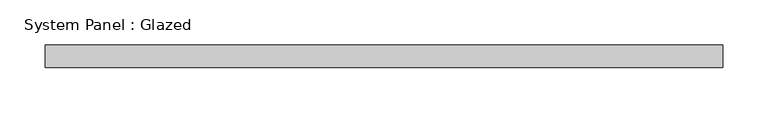
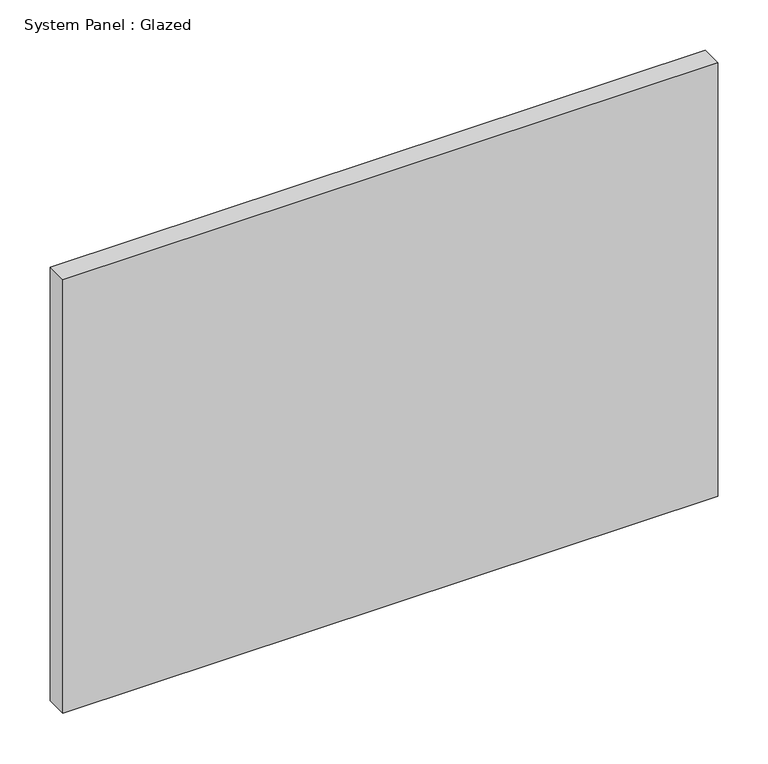
"""IFC4 building model written with IfcOpenShell, lengths in millimetres: plate geometry, System Panel : Glazed."""

from ifc_helpers import new_model, si_unit, origin, origin_with_axes, place, context, project, spatial, polyline, outline, extrude, source, transform, mapped, element, save


def system_panel_glazed_62604723(model_context):
    return source(origin(), model_context, "Body", "SweptSolid", [
        extrude(outline(polyline([(375.0, 24.5), (-375.0, 24.5), (-375.0, 49.5), (375.0, 49.5), (375.0, 24.5)])), origin_with_axes(), (0.0, 0.0, 1.0), 525.0),
    ])


if __name__ == "__main__":
    model = new_model("IFC4")
    model_context = context("Model", 3, world=origin())
    ifc_project = project(units=[si_unit("LENGTHUNIT", "METRE", prefix="MILLI")], contexts=[model_context])
    site = spatial("IfcSite", under=ifc_project)
    building = spatial("IfcBuilding", under=site)
    placement = place(None, origin())
    system_panel_glazed_shape = system_panel_glazed_62604723(model_context)
    element("IfcPlate", 1, ObjectType="System Panel : Glazed", at=placement, inside=building, context=model_context, shape_type="MappedRepresentation", body=[
        mapped(system_panel_glazed_shape, transform((0.0, 0.0, 0.0), x_axis=(1.0, 0.0, 0.0), y_axis=(0.0, 1.0, 0.0), z_axis=(0.0, 0.0, 1.0))),
    ])
    save(model, "model.ifc")

# Revit data of these elements
# Type "System Panel : Glazed"
#   Construction Type Id = "GSP4R"
#   Analytic Construction = "1/8 in Pilkington single glazing"
#   Visual Light Transmittance = 0.9
#   Solar Heat Gain Coefficient = 0.86
#   Heat Transfer Coefficient (U) = 6.7069 W/(m²·K)
#   Define Thermal Properties by = 1
# Element 1 (IfcPlate, "System Panel : Glazed")
#   Materials on its faces: "Glass"
# Materials
#   "Glass": class "Glass", colour RGB 245 245 243, transparency 1, Description = "Soda Lime Glass", Cost = 0
